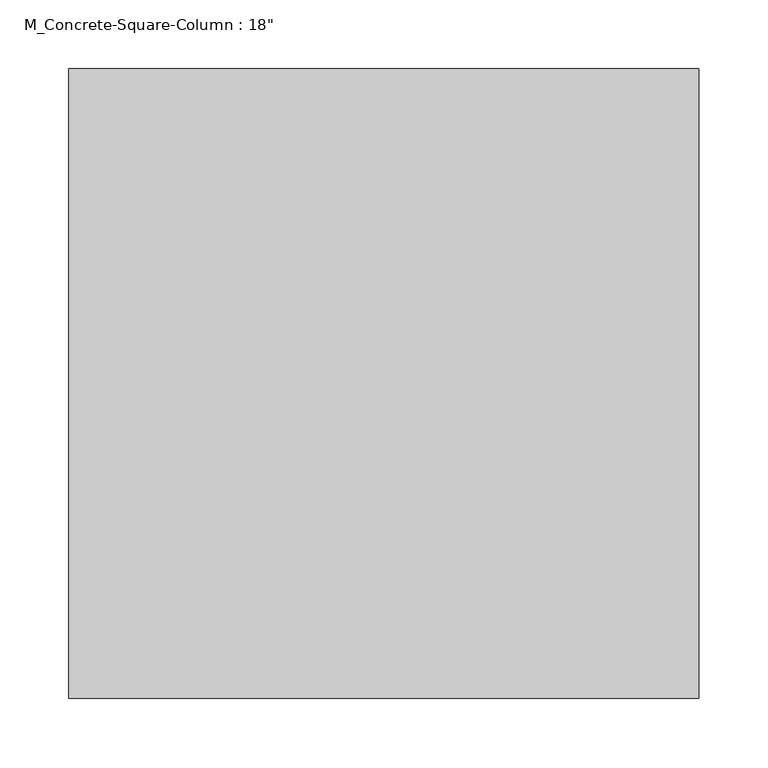
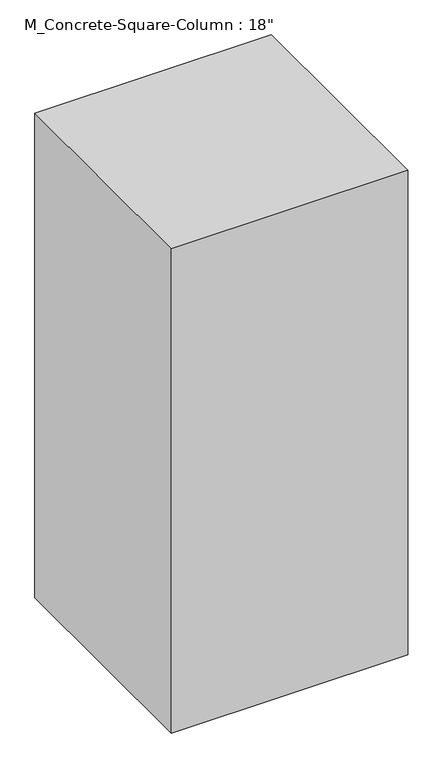
"""IFC4 building model written with IfcOpenShell, lengths in millimetres: column geometry."""

from ifc_helpers import new_model, si_unit, frame, origin, place, context, project, spatial, polyline, outline, extrude, source, transform, mapped, element, save


def column_547059a2(model_context):
    return source(origin(), model_context, "Body", "SweptSolid", [
        extrude(outline(polyline([(228.6, 228.6), (228.6, -228.6), (-228.6, -228.6), (-228.6, 228.6), (228.6, 228.6)])), frame((0.0, 0.0, -2133.6), z_axis=(0.0, 0.0, 1.0), x_axis=(1.0, 0.0, 0.0)), (0.0, 0.0, 1.0), 990.6),
    ])


if __name__ == "__main__":
    model = new_model("IFC4")
    model_context = context("Model", 3, world=origin())
    ifc_project = project(units=[si_unit("LENGTHUNIT", "METRE", prefix="MILLI")], contexts=[model_context])
    site = spatial("IfcSite", under=ifc_project)
    building = spatial("IfcBuilding", under=site)
    placement = place(None, origin())
    column_shape = column_547059a2(model_context)
    element("IfcColumn", 1, ObjectType="M_Concrete-Square-Column : 18\"", at=placement, inside=building, context=model_context, shape_type="MappedRepresentation", body=[
        mapped(column_shape, transform((0.0, 0.0, 0.0), x_axis=(1.0, 0.0, 0.0), y_axis=(0.0, 1.0, 0.0), z_axis=(0.0, 0.0, 1.0))),
    ])
    save(model, "model.ifc")

# Revit data of these elements
# Type "M_Concrete-Square-Column : 18\""
#   b = 457.2 mm
#   Structural Material [instance default] = Concrete, Cast-in-Place gray
# Element 1 (IfcColumn, "M_Concrete-Square-Column : 18\"")
#   Materials on its faces: "Concrete, Cast-in-Place gray"
# Materials
#   "Concrete, Cast-in-Place gray": class "Concrete", colour RGB 192 192 192, transparency 0, Description = "Cast-in-place concrete", Cost = 0
